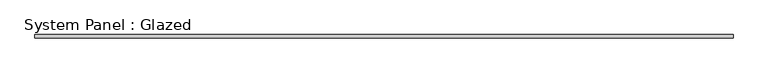
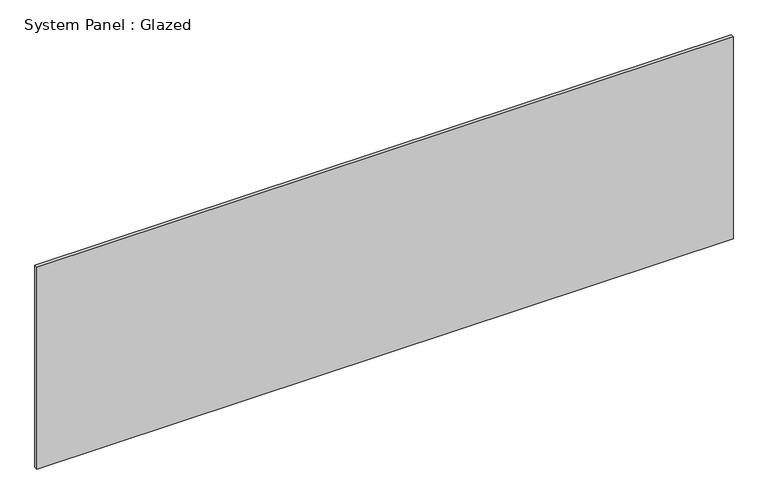
"""IFC4 building model written with IfcOpenShell, lengths in millimetres: plate geometry, System Panel : Glazed."""

from ifc_helpers import new_model, si_unit, origin, origin_with_axes, place, context, project, spatial, polyline, outline, extrude, source, transform, mapped, element, save


def system_panel_glazed_64af9de3(model_context):
    return source(origin(), model_context, "Body", "SweptSolid", [
        extrude(outline(polyline([(2489.2, 19.05), (-2489.2, 19.05), (-2489.2, 44.45), (2489.2, 44.45), (2489.2, 19.05)])), origin_with_axes(), (0.0, 0.0, 1.0), 1524.0),
    ])


if __name__ == "__main__":
    model = new_model("IFC4")
    model_context = context("Model", 3, world=origin())
    ifc_project = project(units=[si_unit("LENGTHUNIT", "METRE", prefix="MILLI")], contexts=[model_context])
    site = spatial("IfcSite", under=ifc_project)
    building = spatial("IfcBuilding", under=site)
    placement = place(None, origin())
    system_panel_glazed_shape = system_panel_glazed_64af9de3(model_context)
    element("IfcPlate", 1, ObjectType="System Panel : Glazed", at=placement, inside=building, context=model_context, shape_type="MappedRepresentation", body=[
        mapped(system_panel_glazed_shape, transform((0.0, 0.0, 0.0), x_axis=(1.0, 0.0, 0.0), y_axis=(0.0, 1.0, 0.0), z_axis=(0.0, 0.0, 1.0))),
    ])
    save(model, "model.ifc")

# Revit data of these elements
# Type "System Panel : Glazed"
#   Construction Type Id = "GSP4R"
#   Analytic Construction = "1/8 in Pilkington single glazing"
#   Visual Light Transmittance = 0.9
#   Solar Heat Gain Coefficient = 0.86
#   Heat Transfer Coefficient (U) = 1.18115 BTU/(h·ft²·°F)
# Element 1 (IfcPlate, "System Panel : Glazed")
#   Materials on its faces: "Glass"
# Materials
#   "Glass": class "Glass", colour RGB 0 128 192, transparency 0.75, Description = "Soda Lime Glass", Cost = 0
